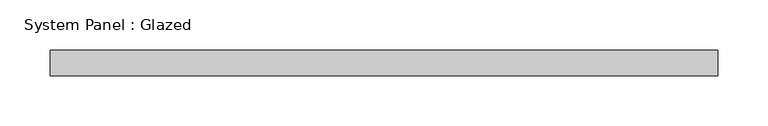
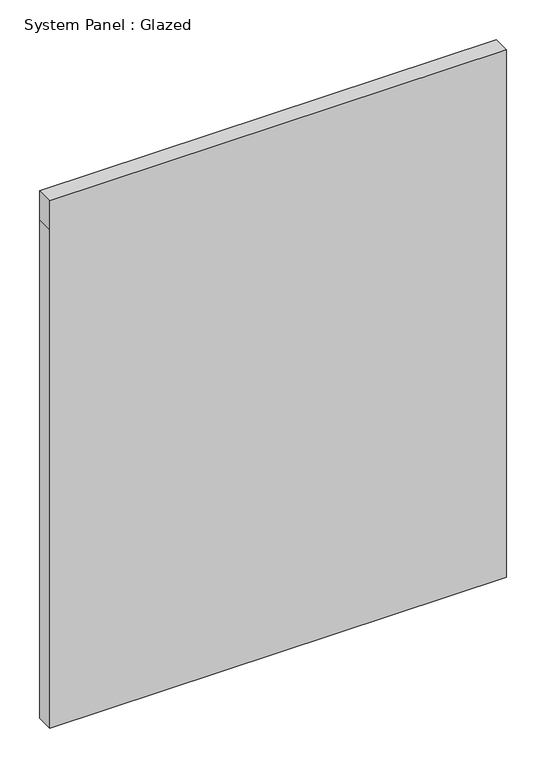
"""IFC4 building model written with IfcOpenShell, lengths in millimetres: plate geometry, System Panel : Glazed."""

from ifc_helpers import new_model, si_unit, frame, origin, place, context, project, spatial, polyline, outline, extrude, source, transform, mapped, element, save


def system_panel_glazed_0a1fe405(model_context):
    return source(origin(), model_context, "Body", "SweptSolid", [
        extrude(outline(polyline([(0.0, -333.375), (0.0, 333.375), (768.9388769, 333.375), (813.3888769, 333.375), (813.3888769, -333.375), (768.9388769, -333.375), (0.0, -333.375)])), frame((0.0, 19.05, 0.0), z_axis=(0.0, 1.0, 0.0), x_axis=(0.0, 0.0, 1.0)), (0.0, 0.0, 1.0), 25.4),
    ])


if __name__ == "__main__":
    model = new_model("IFC4")
    model_context = context("Model", 3, world=origin())
    ifc_project = project(units=[si_unit("LENGTHUNIT", "METRE", prefix="MILLI")], contexts=[model_context])
    site = spatial("IfcSite", under=ifc_project)
    building = spatial("IfcBuilding", under=site)
    placement = place(None, origin())
    system_panel_glazed_shape = system_panel_glazed_0a1fe405(model_context)
    element("IfcPlate", 1, ObjectType="System Panel : Glazed", at=placement, inside=building, context=model_context, shape_type="MappedRepresentation", body=[
        mapped(system_panel_glazed_shape, transform((0.0, 0.0, 0.0), x_axis=(1.0, 0.0, 0.0), y_axis=(0.0, 1.0, 0.0), z_axis=(0.0, 0.0, 1.0))),
    ])
    save(model, "model.ifc")

# Revit data of these elements
# Type "System Panel : Glazed"
#   Construction Type Id = "GSP4R"
#   Analytic Construction = "1/8 in Pilkington single glazing"
#   Visual Light Transmittance = 0.9
#   Solar Heat Gain Coefficient = 0.86
#   Heat Transfer Coefficient (U) = 1.18115 BTU/(h·ft²·°F)
#   Define Thermal Properties by = 1
# Element 1 (IfcPlate, "System Panel : Glazed")
#   Materials on its faces: "Glass"
# Materials
#   "Glass": class "Glass", colour RGB 0 128 192, transparency 0.75, Description = "Soda Lime Glass", Cost = 0
